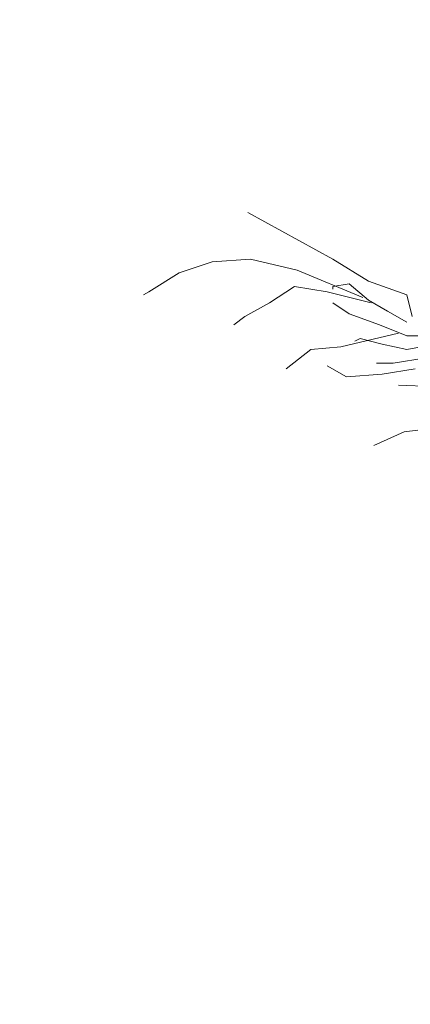
# Model space of a CAD drawing. Units: millimetres. Extents: x 595116 to 630915, y 909473 to 920225.
# Tile 71 of 134: x 629618.945 to 629622.585, y 919276.713 to 919285.898. Entities that reach past the tile are written whole.
import ezdxf

# ---------------------------------------------------------------- set-up
doc = ezdxf.new("R2010")
doc.units = ezdxf.units.MM
doc.layers.add('Dimension', color=3, linetype='Continuous', lineweight=18)
doc.layers.add('L-PLNT', color=85, linetype='Continuous', lineweight=13)
doc.styles.get("Standard").update_dxf_attribs({"font": 'arial.ttf'})
doc.dimstyles.new('ISO-25', dxfattribs={"dimtxt": 9, "dimasz": 6, "dimexe": 1.25, "dimexo": 0.625, "dimtad": 1, "dimlunit": 4, "dimtxsty": 'Standard', "dimcen": 2.5, "dimadec": 0, "dimazin": 0, "dimtfac": 1, "dimtmove": 0, "dimatfit": 3, "dimfxl": 1, "dimarcsym": 0})

# ---------------------------------------------------------------- blocks, each defined once
blk = doc.blocks.new('A$C4FB75ABC')
for p, q in [((0.4999, 4.2779), (0.7111, 4.1621)), ((0.5068, 4.1621), (0.4114, 4.1553)), ((0.6226, 4.1349), (0.5068, 4.1621)), ((0.7111, 4.1621), (0.7997, 4.1076)), ((0.4114, 4.1553), (0.3296, 4.1281)), ((0.3296, 4.1281), (0.2547, 4.0804)), ((0.7861, 4.0668), (0.6226, 4.1349)), ((0.6158, 4.094), (0.5544, 4.0532)), ((0.6975, 4.0804), (0.6158, 4.094)), ((0.752, 4.1008), (0.7111, 4.094)), ((0.7111, 4.094), (0.7111, 4.0872)), ((0.7997, 4.06), (0.752, 4.1008)), ((0.7997, 4.1076), (0.8951, 4.0736)), ((0.2547, 4.0804), (0.241, 4.0736)), ((0.8065, 4.0532), (0.6975, 4.0804)), ((0.8951, 4.0736), (0.9087, 4.0191)), ((0.5544, 4.0532), (0.4931, 4.0191)), ((0.7111, 4.0532), (0.752, 4.0259)), ((0.8474, 4.0327), (0.7997, 4.06)), ((0.4931, 4.0191), (0.4659, 3.9987)), ((0.752, 4.0259), (0.827, 3.9987)), ((0.8951, 4.0055), (0.8474, 4.0327)), ((0.827, 3.9987), (0.8951, 3.9715)), ((0.8746, 3.9783), (0.7316, 3.9442)), ((0.8951, 3.9715), (0.9428, 3.9715)), ((0.7316, 3.9442), (0.6566, 3.9374)), ((0.7793, 3.9647), (0.7656, 3.9578)), ((0.8338, 3.951), (0.7793, 3.9647)), ((0.8951, 3.9374), (0.8338, 3.951)), ((0.97, 3.951), (0.8951, 3.9374)), ((0.6566, 3.9374), (0.5953, 3.8897)), ((0.9428, 3.917), (0.861, 3.9034)), ((0.7452, 3.8693), (0.6975, 3.8966)), ((0.861, 3.9034), (0.8201, 3.9034)), ((0.8338, 3.8761), (0.7452, 3.8693)), ((0.9155, 3.8897), (0.8338, 3.8761)), ((0.8746, 3.8489), (1.0518, 3.8421)), ((0.8133, 3.6991), (0.8883, 3.7331)), ((0.8883, 3.7331), (0.9496, 3.7399))]:
    blk.add_line(p, q)
blk = doc.blocks.new('*D216')
at = {"layer": 'Defpoints', "color": 0, "transparency": 16777216}
for p in [(629743.5408, 919411.9276), (629505.0408, 919411.8279), (629743.5408, 918832.3776)]:
    blk.add_point(p, dxfattribs=at)
at = {"layer": 'Dimension', "color": 0, "lineweight": -2, "transparency": 16777216}
for p, q in [((629743.5408, 919411.3026), (629743.5408, 918831.1276)), ((629505.0408, 919411.2029), (629505.0408, 918831.1276)), ((629511.0408, 918832.3776), (629737.5408, 918832.3776))]:
    blk.add_line(p, q, dxfattribs=at)
at = {"layer": 'Dimension', "color": 0, "transparency": 16777216}
for points in [[(629511.0408, 918833.3776), (629511.0408, 918831.3776), (629505.0408, 918832.3776)], [(629737.5408, 918833.3776), (629737.5408, 918831.3776), (629743.5408, 918832.3776)]]:
    blk.add_solid(points, dxfattribs=at)
at = {"layer": 'Dimension', "color": 0, "transparency": 16777216, "insert": (629624.2908, 918837.656), "char_height": 9, "attachment_point": 5}
blk.add_mtext('19\'-10 1/2"', dxfattribs=at)

msp = doc.modelspace()

# ---------------------------------------------------------------- block references
at = {"layer": 'L-PLNT', "xscale": 3.753413438031968, "yscale": 3.753413438031968, "zscale": 3.753413438031968}
msp.add_blockref('A$C4FB75ABC', (629619.1929, 919268.043), dxfattribs=at)

# ---------------------------------------------------------------- dimensions: what is measured, and where the dimension line sits
at = {"layer": 'Dimension'}
dim = msp.add_linear_dim(base=(629743.5408, 918832.3776), p1=(629505.0408, 919411.8279), p2=(629743.5408, 919411.9276), dimstyle='ISO-25', override={"dimdec": 1, "dimlfac": 1, "dimrnd": 0, "dimzin": 1, "dimdsep": 46, "dimlunit": 4, "dimfrac": 2}, dxfattribs=at)
dim.commit()
dim.dimension.update_dxf_attribs({"geometry": '*D216', "text_midpoint": (629624.2908, 918837.656)})

doc.saveas('drawing.dxf')
